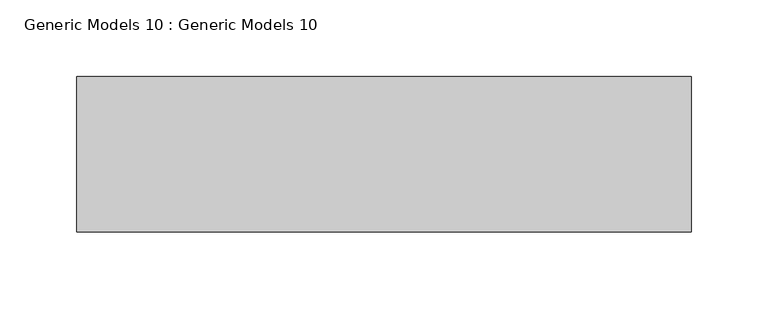
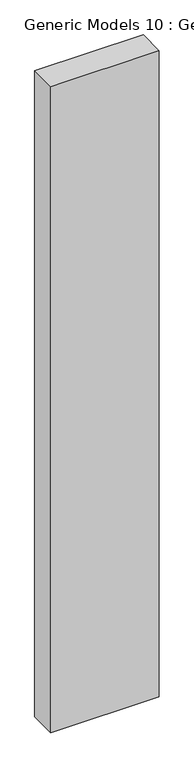
"""IFC4 building model written with IfcOpenShell, lengths in millimetres: proxy geometry, Generic Models 10 : Generic Models 10."""

from ifc_helpers import new_model, si_unit, frame, origin, place, context, project, spatial, polyline, outline, extrude, source, transform, mapped, element, save


def generic_models_10_generic_models_10_d7661e71(model_context):
    return source(origin(), model_context, "Body", "SweptSolid", [
        extrude(outline(polyline([(-4714.5770642, -10372.9896616), (-5116.1972155, -10372.9896616), (-5116.1972155, -10271.3896616), (-4714.5770642, -10271.3896616), (-4714.5770642, -10372.9896616)])), frame((0.0, 0.0, 304.8), z_axis=(0.0, 0.0, 1.0), x_axis=(1.0, 0.0, 0.0)), (0.0, 0.0, 1.0), 2526.2992593),
    ])


if __name__ == "__main__":
    model = new_model("IFC4")
    model_context = context("Model", 3, world=origin())
    ifc_project = project(units=[si_unit("LENGTHUNIT", "METRE", prefix="MILLI")], contexts=[model_context])
    site = spatial("IfcSite", under=ifc_project)
    building = spatial("IfcBuilding", under=site)
    placement = place(None, origin())
    generic_models_10_generic_models_10_shape = generic_models_10_generic_models_10_d7661e71(model_context)
    element("IfcBuildingElementProxy", 1, Name="Generic Models 10 : Generic Models 10", ObjectType="Generic Models 10 : Generic Models 10", at=placement, inside=building, context=model_context, shape_type="MappedRepresentation", body=[
        mapped(generic_models_10_generic_models_10_shape, transform((0.0, 0.0, 0.0), x_axis=(1.0, 0.0, 0.0), y_axis=(0.0, 1.0, 0.0), z_axis=(0.0, 0.0, 1.0))),
    ])
    save(model, "model.ifc")

# Revit data of these elements
# Element 1 (IfcBuildingElementProxy, "Generic Models 10 : Generic Models 10")
#   Materials on its faces: "ACCENT BEIGE COLOUR"
# Materials
#   "ACCENT BEIGE COLOUR": class "Generic", colour RGB 120 120 120, transparency 0, Cost = 0
